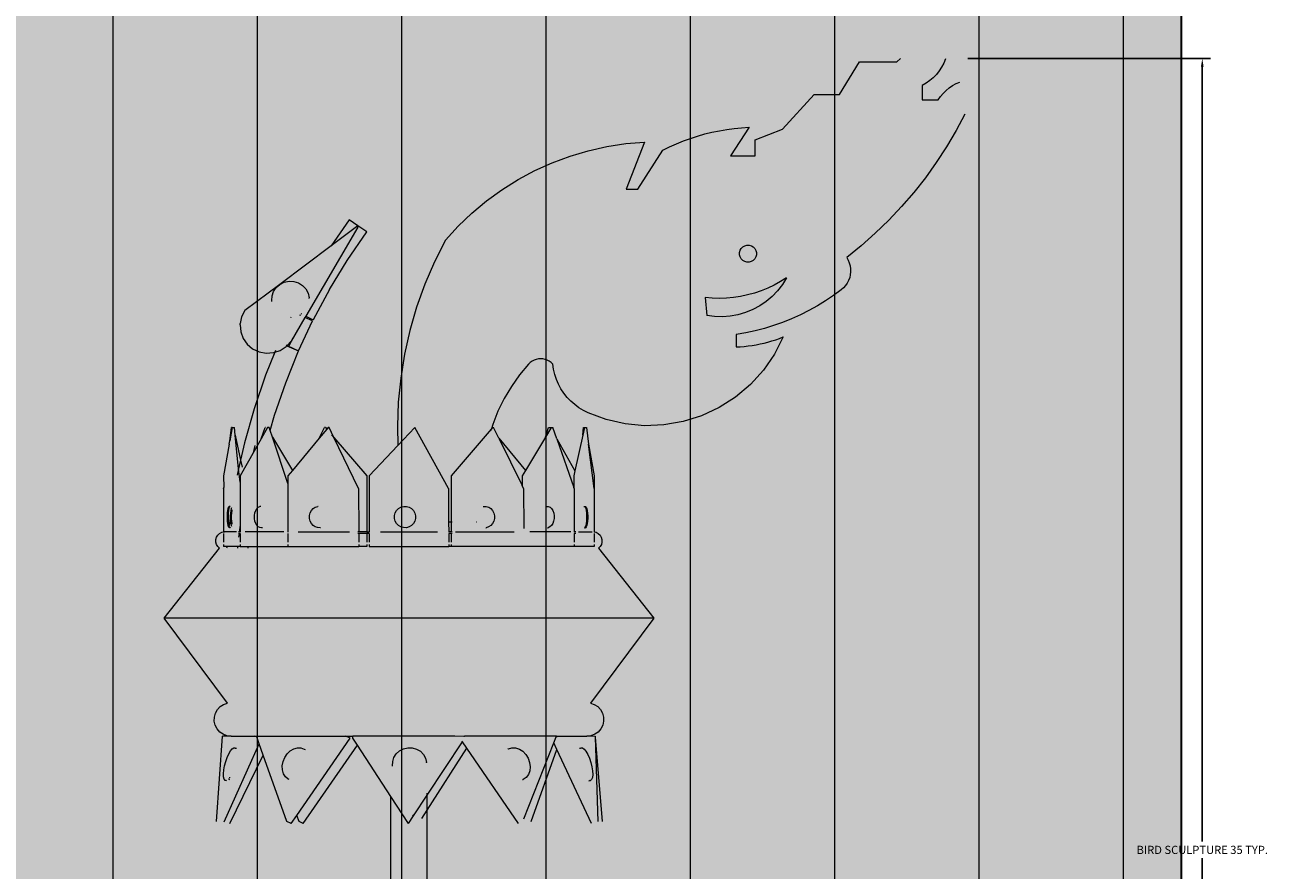
# Model space of a CAD drawing. Units: millimetres. Extents: x 446512 to 447461, y 70395 to 70610.
# Tile 36 of 39: x 447401 to 447428, y 70453 to 70472. Entities that reach past the tile are written whole.
import ezdxf

# ---------------------------------------------------------------- set-up
doc = ezdxf.new("R2010")
doc.units = ezdxf.units.MM
for name, color, linetype, lineweight in [('A-ANNO-DIMS', 2, 'Continuous', 18), ('A-FURN', 7, 'Continuous', 35), ('A-FURN-DECO', 8, 'Continuous', 13), ('A-FURN-PATT', 38, 'Continuous', 13)]:
    doc.layers.add(name, color=color, linetype=linetype, lineweight=lineweight)
doc.styles.get("Standard").update_dxf_attribs({"font": 'arial.ttf'})
doc.dimstyles.get("Standard").update_dxf_attribs({"dimtxt": 0.18, "dimasz": 0.18, "dimexe": 0.18, "dimexo": 0.0625, "dimgap": 0.09, "dimtad": 0, "dimtih": 1, "dimtoh": 1, "dimdec": 4, "dimzin": 0, "dimdsep": 46, "dimtxsty": 'Standard', "dimcen": 0.09, "dimadec": 0, "dimazin": 0, "dimtfac": 1, "dimtdec": 4, "dimtofl": 0, "dimtmove": 0, "dimatfit": 3, "dimfxl": 1, "dimtolj": 1, "dimtzin": 0, "dimarcsym": 0})

# ---------------------------------------------------------------- blocks, each defined once
blk = doc.blocks.new('DECO-SCULPTURE-BIRD')
for p, q in [((15.181, 34.03), (15.627, 34.749)), ((15.627, 34.749), (16.449, 34.749)), ((16.449, 34.749), (16.526, 34.819)), ((13.93, 33.268), (14.629, 34.03)), ((14.629, 34.03), (15.181, 34.03)), ((17.942, 33.598), (17.748, 33.234)), ((11.904, 33.064), (12.061, 33.115)), ((12.061, 33.115), (12.219, 33.16)), ((12.219, 33.16), (12.379, 33.199)), ((12.379, 33.199), (12.541, 33.233)), ((12.541, 33.233), (12.703, 33.261)), ((12.703, 33.261), (12.866, 33.283)), ((13.195, 33.309), (12.789, 32.676)), ((12.866, 33.283), (13.03, 33.299)), ((13.03, 33.299), (13.195, 33.309)), ((13.33, 33.029), (13.93, 33.268)), ((17.748, 33.234), (17.539, 32.879)), ((9.658, 32.793), (10.067, 32.884)), ((10.067, 32.884), (10.481, 32.948)), ((10.481, 32.948), (10.898, 32.983)), ((10.898, 32.983), (10.488, 31.945)), ((10.747, 31.945), (11.298, 32.806)), ((11.298, 32.806), (11.446, 32.878)), ((11.446, 32.878), (11.597, 32.946)), ((11.597, 32.946), (11.749, 33.008)), ((11.749, 33.008), (11.904, 33.064)), ((13.33, 32.676), (13.33, 33.029)), ((17.539, 32.879), (17.314, 32.533)), ((8.482, 32.355), (8.864, 32.528)), ((8.864, 32.528), (9.257, 32.674)), ((9.257, 32.674), (9.658, 32.793)), ((12.789, 32.676), (13.33, 32.676)), ((17.314, 32.533), (17.074, 32.198)), ((8.113, 32.157), (8.482, 32.355)), ((7.759, 31.935), (8.113, 32.157)), ((17.074, 32.198), (16.819, 31.874)), ((7.42, 31.689), (7.759, 31.935)), ((10.488, 31.945), (10.747, 31.945)), ((16.819, 31.874), (16.55, 31.562)), ((7.098, 31.42), (7.42, 31.689)), ((16.55, 31.562), (16.267, 31.262)), ((4.396, 31.274), (4.005, 30.703)), ((4.59, 31.141), (4.396, 31.274)), ((6.796, 31.131), (7.098, 31.42)), ((16.267, 31.262), (15.971, 30.975)), ((4.59, 31.11), (3.442, 29.152)), ((4.59, 31.141), (4.005, 30.703)), ((4.354, 30.38), (4.784, 31.008)), ((4.59, 31.11), (4.59, 31.141)), ((4.784, 31.008), (4.59, 31.141)), ((6.514, 30.821), (6.796, 31.131)), ((15.971, 30.975), (15.663, 30.701)), ((4.005, 30.703), (2.875, 29.852)), ((6.514, 30.821), (6.273, 30.344)), ((15.663, 30.701), (15.342, 30.442)), ((3.962, 29.736), (4.354, 30.38)), ((6.273, 30.344), (6.062, 29.854)), ((15.342, 30.442), (15.375, 30.385)), ((15.375, 30.385), (15.4, 30.324)), ((15.4, 30.324), (15.418, 30.261)), ((15.422, 30.065), (15.408, 30.001)), ((15.418, 30.261), (15.428, 30.196)), ((15.429, 30.13), (15.422, 30.065)), ((15.428, 30.196), (15.429, 30.13)), ((2.875, 29.852), (2.1, 29.278)), ((2.795, 29.783), (2.875, 29.852)), ((2.875, 29.852), (2.971, 29.899)), ((2.971, 29.899), (3.076, 29.921)), ((3.076, 29.921), (3.183, 29.915)), ((3.183, 29.915), (3.285, 29.883)), ((3.285, 29.883), (3.375, 29.827)), ((3.375, 29.827), (3.447, 29.75)), ((6.062, 29.854), (5.881, 29.351)), ((15.318, 29.827), (15.274, 29.778)), ((15.355, 29.881), (15.318, 29.827)), ((15.385, 29.939), (15.355, 29.881)), ((15.408, 30.001), (15.385, 29.939)), ((2.698, 29.494), (2.704, 29.597)), ((2.704, 29.597), (2.737, 29.696)), ((2.737, 29.696), (2.795, 29.783)), ((3.447, 29.75), (3.496, 29.657)), ((3.496, 29.657), (3.518, 29.556)), ((3.517, 29.541), (3.518, 29.556)), ((3.517, 29.541), (3.518, 29.538)), ((3.962, 29.736), (3.605, 29.071)), ((15.054, 29.609), (14.878, 29.491)), ((15.224, 29.735), (15.054, 29.609)), ((15.274, 29.778), (15.224, 29.735)), ((2.1, 29.278), (2.031, 29.139)), ((2.699, 29.49), (2.698, 29.494)), ((2.698, 29.476), (2.699, 29.49)), ((5.881, 29.351), (5.732, 28.838)), ((14.513, 29.277), (14.324, 29.181)), ((14.698, 29.38), (14.513, 29.277)), ((14.878, 29.491), (14.698, 29.38)), ((2.031, 29.139), (2.002, 28.989)), ((2.002, 28.958), (2.002, 28.989)), ((3.425, 29.125), (3.119, 28.602)), ((3.287, 28.392), (3.593, 29.046)), ((3.306, 29.18), (3.325, 29.171)), ((3.358, 29.194), (3.345, 29.201)), ((3.442, 29.152), (3.425, 29.125)), ((3.593, 29.046), (3.425, 29.125)), ((3.442, 29.152), (3.605, 29.071)), ((13.934, 29.015), (13.735, 28.944)), ((14.131, 29.094), (13.934, 29.015)), ((14.324, 29.181), (14.131, 29.094)), ((2.002, 28.958), (2.013, 28.805)), ((2.013, 28.805), (2.066, 28.66)), ((5.732, 28.838), (5.615, 28.317)), ((13.121, 28.783), (12.912, 28.746)), ((12.912, 28.746), (12.912, 28.476)), ((13.328, 28.828), (13.121, 28.783)), ((13.532, 28.882), (13.328, 28.828)), ((13.735, 28.944), (13.532, 28.882)), ((13.947, 28.695), (13.752, 28.315)), ((13.864, 28.663), (13.947, 28.695)), ((2.066, 28.66), (2.155, 28.533)), ((2.155, 28.533), (2.275, 28.433)), ((2.275, 28.433), (2.419, 28.366)), ((2.883, 28.399), (3.015, 28.486)), ((3.005, 28.509), (3.027, 28.499)), ((3.015, 28.486), (3.027, 28.499)), ((3.036, 28.509), (3.019, 28.518)), ((3.027, 28.499), (3.036, 28.509)), ((3.027, 28.499), (3.284, 28.387)), ((3.036, 28.509), (3.119, 28.602)), ((3.036, 28.509), (3.287, 28.392)), ((3.074, 28.492), (3.069, 28.481)), ((3.152, 28.659), (3.074, 28.492)), ((12.912, 28.476), (13.001, 28.48)), ((13.001, 28.48), (13.089, 28.487)), ((13.089, 28.487), (13.177, 28.496)), ((13.177, 28.496), (13.265, 28.508)), ((13.265, 28.508), (13.352, 28.523)), ((13.352, 28.523), (13.439, 28.54)), ((13.439, 28.54), (13.525, 28.559)), ((13.525, 28.559), (13.611, 28.581)), ((13.611, 28.581), (13.696, 28.606)), ((13.696, 28.606), (13.781, 28.633)), ((13.781, 28.633), (13.864, 28.663)), ((2.419, 28.366), (2.575, 28.337)), ((2.766, 28.36), (2.561, 27.852)), ((2.575, 28.337), (2.733, 28.349)), ((2.733, 28.349), (2.766, 28.36)), ((2.766, 28.36), (2.883, 28.399)), ((2.781, 28.395), (2.766, 28.36)), ((3.002, 27.688), (3.284, 28.387)), ((5.615, 28.317), (5.531, 27.79)), ((8.422, 28.162), (8.382, 28.133)), ((8.466, 28.185), (8.422, 28.162)), ((8.513, 28.202), (8.466, 28.185)), ((8.561, 28.212), (8.513, 28.202)), ((8.611, 28.216), (8.561, 28.212)), ((8.66, 28.212), (8.611, 28.216)), ((8.709, 28.202), (8.66, 28.212)), ((8.756, 28.185), (8.709, 28.202)), ((8.799, 28.162), (8.756, 28.185)), ((8.84, 28.133), (8.799, 28.162)), ((13.752, 28.315), (13.509, 27.964)), ((8.346, 28.098), (8.147, 27.859)), ((8.382, 28.133), (8.346, 28.098)), ((8.875, 28.098), (8.84, 28.133)), ((8.892, 27.984), (8.875, 28.098)), ((8.919, 27.871), (8.892, 27.984)), ((13.509, 27.964), (13.223, 27.648)), ((2.561, 27.852), (2.308, 27.114)), ((2.757, 26.974), (3.002, 27.688)), ((5.531, 27.79), (5.479, 27.259)), ((7.968, 27.605), (7.808, 27.338)), ((8.147, 27.859), (7.968, 27.605)), ((8.956, 27.761), (8.919, 27.871)), ((9.002, 27.655), (8.956, 27.761)), ((9.057, 27.553), (9.002, 27.655)), ((13.223, 27.648), (12.897, 27.372)), ((7.808, 27.338), (7.671, 27.059)), ((9.121, 27.456), (9.057, 27.553)), ((9.193, 27.366), (9.121, 27.456)), ((9.273, 27.282), (9.193, 27.366)), ((12.897, 27.372), (12.537, 27.142)), ((2.308, 27.114), (2.095, 26.364)), ((5.479, 27.259), (5.46, 26.725)), ((7.671, 27.059), (7.556, 26.77)), ((9.359, 27.205), (9.273, 27.282)), ((9.452, 27.136), (9.359, 27.205)), ((9.551, 27.075), (9.452, 27.136)), ((9.654, 27.023), (9.551, 27.075)), ((12.537, 27.142), (12.15, 26.961)), ((2.662, 26.638), (2.757, 26.974)), ((10.055, 26.875), (9.654, 27.023)), ((10.471, 26.78), (10.055, 26.875)), ((11.743, 26.833), (11.323, 26.759)), ((12.15, 26.961), (11.743, 26.833)), ((1.77, 26.41), (1.808, 26.703)), ((1.827, 26.703), (1.77, 26.41)), ((1.827, 26.703), (1.808, 26.703)), ((1.827, 26.703), (1.873, 26.703)), ((1.89, 26.535), (1.873, 26.703)), ((1.89, 26.535), (2.01, 25.987)), ((1.967, 25.795), (1.89, 26.535)), ((2.459, 26.45), (2.547, 26.703)), ((2.603, 26.703), (2.459, 26.45)), ((2.558, 26.703), (2.547, 26.703)), ((2.64, 26.703), (2.603, 26.703)), ((2.662, 26.638), (2.64, 26.703)), ((2.709, 26.493), (2.662, 26.638)), ((3.737, 26.466), (3.854, 26.703)), ((3.905, 26.667), (3.737, 26.466)), ((3.875, 26.703), (3.854, 26.703)), ((3.875, 26.703), (3.905, 26.667)), ((3.935, 26.703), (3.905, 26.667)), ((3.957, 26.703), (3.935, 26.703)), ((4.064, 26.48), (3.957, 26.703)), ((4.013, 26.541), (4.064, 26.48)), ((5.46, 26.725), (5.471, 26.308)), ((5.845, 26.703), (5.471, 26.308)), ((6.58, 25.364), (5.845, 26.703)), ((7.523, 26.665), (6.643, 25.636)), ((7.523, 26.665), (7.514, 26.636)), ((7.526, 26.673), (7.523, 26.665)), ((7.523, 26.665), (7.531, 26.655)), ((7.556, 26.77), (7.526, 26.673)), ((7.551, 26.703), (7.526, 26.673)), ((7.551, 26.703), (7.572, 26.703)), ((7.688, 26.466), (7.572, 26.703)), ((8.717, 26.493), (8.786, 26.703)), ((8.833, 26.686), (8.717, 26.493)), ((8.786, 26.703), (8.823, 26.703)), ((8.823, 26.703), (8.833, 26.686)), ((8.843, 26.703), (8.833, 26.686)), ((8.843, 26.703), (8.879, 26.703)), ((8.967, 26.45), (8.879, 26.703)), ((9.536, 26.535), (9.364, 25.75)), ((9.536, 26.535), (9.553, 26.703)), ((9.573, 26.703), (9.536, 26.535)), ((9.553, 26.703), (9.573, 26.703)), ((9.573, 26.703), (9.618, 26.703)), ((9.618, 26.703), (9.665, 26.337)), ((10.896, 26.742), (10.471, 26.78)), ((11.323, 26.759), (10.896, 26.742)), ((1.761, 26.337), (1.636, 25.636)), ((1.761, 26.337), (1.77, 26.41)), ((2.459, 26.45), (1.998, 25.636)), ((2.095, 26.364), (2.01, 25.987)), ((2.709, 26.493), (3.149, 25.76)), ((3.046, 25.467), (2.709, 26.493)), ((3.737, 26.466), (3.149, 25.76)), ((4.064, 26.48), (4.783, 25.636)), ((4.603, 25.364), (4.064, 26.48)), ((5.471, 26.308), (4.835, 25.636)), ((7.688, 26.466), (8.277, 25.76)), ((7.688, 26.466), (8.203, 25.423)), ((8.717, 26.493), (8.277, 25.76)), ((8.967, 26.45), (9.364, 25.75)), ((8.967, 26.45), (9.339, 25.38)), ((9.665, 26.337), (9.79, 25.636)), ((9.789, 25.364), (9.665, 26.337)), ((2.01, 25.987), (1.967, 25.795)), ((2.01, 25.987), (2.045, 25.829)), ((1.967, 25.795), (1.935, 25.655)), ((1.998, 25.499), (1.967, 25.795)), ((3.149, 25.76), (3.046, 25.636)), ((8.277, 25.76), (8.203, 25.636)), ((9.364, 25.75), (9.339, 25.636)), ((1.636, 25.636), (1.639, 25.38)), ((1.998, 25.636), (1.998, 25.499)), ((1.998, 25.499), (1.998, 24.41)), ((3.046, 25.636), (3.046, 25.467)), ((3.046, 25.467), (3.046, 24.397)), ((4.783, 25.636), (4.783, 24.41)), ((4.835, 25.636), (4.835, 24.41)), ((6.643, 25.636), (6.643, 24.617)), ((8.203, 25.636), (8.203, 25.423)), ((8.232, 25.364), (8.203, 25.423)), ((9.339, 25.636), (9.339, 25.38)), ((9.79, 25.636), (9.789, 25.364)), ((1.637, 25.364), (1.635, 24.407)), ((1.637, 25.364), (1.639, 25.38)), ((4.603, 25.364), (4.61, 24.41)), ((6.58, 25.364), (6.586, 24.617)), ((8.232, 25.364), (8.239, 24.482)), ((9.344, 25.364), (9.339, 25.38)), ((9.344, 25.364), (9.349, 24.41)), ((9.789, 25.364), (9.79, 24.407)), ((6.643, 24.617), (6.586, 24.617)), ((6.586, 24.617), (6.588, 24.41)), ((6.663, 24.617), (6.643, 24.617)), ((6.643, 24.617), (6.643, 24.41)), ((1.483, 24.287), (1.51, 24.333)), ((1.51, 24.333), (1.549, 24.371)), ((1.549, 24.371), (1.595, 24.397)), ((1.595, 24.397), (1.635, 24.407)), ((1.635, 24.407), (1.648, 24.41)), ((1.635, 24.407), (1.635, 24.397)), ((1.635, 24.371), (1.635, 24.182)), ((1.648, 24.41), (1.657, 24.41)), ((1.648, 24.41), (1.651, 24.41)), ((1.923, 24.41), (1.657, 24.41)), ((1.998, 24.41), (1.967, 24.41)), ((1.977, 24.371), (1.967, 24.29)), ((1.998, 24.367), (1.967, 24.367)), ((1.998, 24.556), (1.98, 24.397)), ((1.998, 24.41), (1.998, 24.397)), ((1.998, 24.371), (1.998, 24.367)), ((1.998, 24.367), (1.998, 24.182)), ((2.958, 24.41), (2.109, 24.41)), ((3.046, 24.371), (3.046, 24.182)), ((4.61, 24.41), (4.588, 24.41)), ((4.611, 24.367), (4.588, 24.367)), ((4.61, 24.41), (4.611, 24.397)), ((4.783, 24.41), (4.61, 24.41)), ((4.611, 24.371), (4.611, 24.367)), ((4.611, 24.367), (4.612, 24.182)), ((4.783, 24.367), (4.611, 24.367)), ((4.783, 24.41), (4.835, 24.41)), ((4.783, 24.41), (4.783, 24.397)), ((4.783, 24.371), (4.783, 24.367)), ((4.783, 24.367), (4.783, 24.182)), ((4.835, 24.367), (4.783, 24.367)), ((4.835, 24.41), (4.835, 24.397)), ((4.835, 24.371), (4.835, 24.367)), ((4.835, 24.367), (4.835, 24.182)), ((6.588, 24.41), (6.588, 24.397)), ((6.643, 24.41), (6.588, 24.41)), ((6.588, 24.371), (6.588, 24.367)), ((6.588, 24.367), (6.59, 24.182)), ((6.643, 24.367), (6.588, 24.367)), ((6.663, 24.41), (6.643, 24.41)), ((6.643, 24.41), (6.643, 24.397)), ((6.643, 24.371), (6.643, 24.367)), ((6.663, 24.367), (6.643, 24.367)), ((6.643, 24.367), (6.643, 24.182)), ((6.737, 24.41), (8.029, 24.41)), ((9.272, 24.41), (8.372, 24.41)), ((9.384, 24.41), (9.349, 24.41)), ((9.349, 24.41), (9.35, 24.397)), ((9.35, 24.371), (9.35, 24.367)), ((9.384, 24.367), (9.35, 24.367)), ((9.35, 24.367), (9.351, 24.182)), ((9.445, 24.41), (9.742, 24.41)), ((9.79, 24.407), (9.83, 24.397)), ((9.79, 24.407), (9.79, 24.397)), ((9.79, 24.371), (9.79, 24.182)), ((9.83, 24.397), (9.877, 24.371)), ((9.877, 24.371), (9.916, 24.333)), ((9.916, 24.333), (9.943, 24.287)), ((1.467, 24.182), (1.468, 24.235)), ((1.48, 24.13), (1.467, 24.182)), ((1.468, 24.235), (1.483, 24.287)), ((1.507, 24.083), (1.48, 24.13)), ((1.544, 24.044), (1.507, 24.083)), ((1.635, 24.13), (1.635, 24.083)), ((1.639, 24.083), (1.635, 24.083)), ((1.707, 24.083), (1.635, 24.083)), ((1.704, 24.059), (1.703, 24.044)), ((1.707, 24.083), (1.704, 24.059)), ((1.998, 24.083), (1.707, 24.083)), ((1.944, 24.083), (1.939, 24.044)), ((1.998, 24.13), (1.998, 24.083)), ((1.998, 24.083), (2.18, 24.083)), ((2.176, 24.044), (2.18, 24.083)), ((2.18, 24.083), (3.049, 24.083)), ((3.046, 24.13), (3.049, 24.083)), ((3.049, 24.083), (4.613, 24.083)), ((4.613, 24.13), (4.613, 24.083)), ((4.783, 24.083), (4.613, 24.083)), ((4.783, 24.13), (4.783, 24.083)), ((4.835, 24.13), (4.835, 24.083)), ((4.835, 24.083), (6.591, 24.083)), ((6.59, 24.13), (6.591, 24.083)), ((6.643, 24.083), (6.591, 24.083)), ((6.643, 24.13), (6.643, 24.083)), ((9.351, 24.083), (6.643, 24.083)), ((9.351, 24.13), (9.351, 24.083)), ((9.79, 24.083), (9.351, 24.083)), ((9.79, 24.13), (9.79, 24.083)), ((9.919, 24.083), (9.882, 24.044)), ((9.946, 24.13), (9.919, 24.083)), ((9.943, 24.287), (9.958, 24.235)), ((9.959, 24.182), (9.946, 24.13)), ((9.958, 24.235), (9.959, 24.182)), ((0.327, 22.505), (1.544, 24.044)), ((9.882, 24.044), (11.099, 22.505)), ((1.72, 20.641), (0.327, 22.505)), ((11.099, 22.505), (0.327, 22.505)), ((11.099, 22.505), (9.706, 20.641)), ((1.498, 20.496), (1.56, 20.562)), ((1.56, 20.562), (1.635, 20.611)), ((1.635, 20.611), (1.72, 20.641)), ((9.706, 20.641), (9.791, 20.611)), ((9.791, 20.611), (9.866, 20.562)), ((9.866, 20.562), (9.927, 20.496)), ((1.431, 20.239), (1.432, 20.329)), ((1.451, 20.152), (1.431, 20.239)), ((1.432, 20.329), (1.455, 20.417)), ((1.455, 20.417), (1.498, 20.496)), ((9.927, 20.496), (9.971, 20.417)), ((9.971, 20.417), (9.994, 20.329)), ((9.995, 20.239), (9.975, 20.152)), ((9.994, 20.329), (9.995, 20.239)), ((1.492, 20.071), (1.451, 20.152)), ((1.551, 20.003), (1.492, 20.071)), ((1.625, 19.952), (1.551, 20.003)), ((1.709, 19.92), (1.625, 19.952)), ((9.801, 19.952), (9.716, 19.92)), ((9.874, 20.003), (9.801, 19.952)), ((9.934, 20.071), (9.874, 20.003)), ((9.975, 20.152), (9.934, 20.071)), ((1.48, 18.035), (1.609, 19.909)), ((1.799, 19.909), (1.609, 19.909)), ((1.648, 18.028), (2.417, 19.746)), ((1.799, 19.909), (1.709, 19.92)), ((1.799, 19.909), (2.323, 19.909)), ((2.323, 19.909), (2.359, 19.909)), ((2.364, 19.896), (2.323, 19.909)), ((2.364, 19.896), (2.359, 19.909)), ((2.359, 19.909), (4.323, 19.909)), ((2.417, 19.746), (2.364, 19.896)), ((2.508, 19.49), (2.417, 19.746)), ((3.245, 18.169), (4.419, 19.866)), ((3.386, 17.993), (4.578, 19.714)), ((4.323, 19.909), (4.479, 19.909)), ((4.419, 19.866), (4.323, 19.909)), ((4.479, 19.866), (4.479, 19.909)), ((6.726, 19.909), (4.479, 19.909)), ((4.578, 19.714), (4.479, 19.866)), ((5.313, 18.586), (4.578, 19.714)), ((6.112, 18.612), (6.893, 19.784)), ((6.922, 19.907), (6.726, 19.909)), ((6.893, 19.784), (6.878, 19.805)), ((6.985, 19.65), (6.893, 19.784)), ((6.922, 19.907), (6.926, 19.909)), ((6.926, 19.909), (6.936, 19.909)), ((8.957, 19.909), (6.936, 19.909)), ((8.239, 18.093), (8.898, 19.762)), ((8.898, 19.762), (8.95, 19.895)), ((8.967, 19.615), (8.898, 19.762)), ((8.95, 19.895), (8.999, 19.909)), ((8.95, 19.895), (8.957, 19.909)), ((8.957, 19.909), (8.999, 19.909)), ((8.999, 19.909), (9.627, 19.909)), ((9.716, 19.92), (9.627, 19.909)), ((9.807, 19.907), (9.627, 19.909)), ((9.814, 19.909), (9.807, 19.907)), ((9.816, 19.893), (9.814, 19.909)), ((9.974, 18.035), (9.816, 19.893)), ((9.876, 18.035), (9.816, 19.893)), ((1.771, 17.993), (2.508, 19.49)), ((3.027, 18.035), (2.508, 19.49)), ((6.112, 18.284), (6.985, 19.65)), ((8.126, 17.993), (6.985, 19.65)), ((8.405, 18.035), (8.967, 19.615)), ((9.727, 17.993), (8.967, 19.615)), ((5.313, 11.612), (5.313, 18.586)), ((5.7, 17.993), (5.313, 18.586)), ((5.812, 18.161), (6.112, 18.612)), ((6.112, 18.612), (6.112, 18.655)), ((6.112, 18.284), (6.112, 18.612)), ((3.123, 17.993), (3.245, 18.169)), ((3.299, 18.035), (3.245, 18.169)), ((5.7, 17.993), (5.812, 18.161)), ((5.812, 18.161), (5.798, 18.182)), ((5.816, 18.155), (5.812, 18.161)), ((5.995, 18.101), (6.112, 18.284)), ((6.112, 11.612), (6.112, 18.284)), ((3.123, 17.993), (3.027, 18.035)), ((3.386, 17.993), (3.299, 18.035)), ((0, 0), (0, 11.612)), ((0, 11.612), (5.313, 11.612)), ((6.112, 11.612), (5.313, 11.612)), ((6.112, 11.612), (11.751, 11.612)), ((11.751, 0), (11.751, 11.612)), ((0, 0), (11.751, 0))]:
    blk.add_line(p, q)
blk = doc.blocks.new('*D5')
at = {"layer": 'A-ANNO-DIMS', "color": 0, "lineweight": -2, "transparency": 16777216}
for p, q in [((447421.309, 70471.106), (447426.65, 70471.106)), ((447426.47, 70470.926), (447426.47, 70453.88)), ((447426.47, 70436.468), (447426.47, 70453.514)), ((447421.309, 70436.288), (447426.65, 70436.288))]:
    blk.add_line(p, q, dxfattribs=at)
at = {"layer": 'A-ANNO-DIMS', "color": 0, "transparency": 16777216}
for points in [[(447426.44, 70470.926), (447426.5, 70470.926), (447426.47, 70471.106)], [(447426.44, 70436.468), (447426.5, 70436.468), (447426.47, 70436.288)]]:
    blk.add_solid(points, dxfattribs=at)
at = {"layer": 'Defpoints', "color": 0, "transparency": 16777216}
for p in [(447421.247, 70471.106), (447426.47, 70471.106), (447421.247, 70436.288)]:
    blk.add_point(p, dxfattribs=at)
at = {"layer": 'A-ANNO-DIMS', "color": 0, "transparency": 16777216, "insert": (447426.47, 70453.697), "char_height": 0.18, "attachment_point": 5}
blk.add_mtext('\\A1;BIRD SCULPTURE 35 TYP.', dxfattribs=at)

msp = doc.modelspace()

# ---------------------------------------------------------------- hatches: boundary and pattern name
at = {"layer": 'A-FURN-PATT'}
h = msp.add_hatch(dxfattribs=at)
h.set_pattern_fill('ANSI31', color=256, angle=45)
h.set_pattern_definition([(90, (127.5626, 0), (-3.175, 0), [])])
h.paths.add_polyline_path([(447426.0142, 70599.7147), (447365.4251, 70599.7147), (447365.4251, 70405.3145), (447426.0142, 70405.3145)])
h = msp.add_hatch(color=256, dxfattribs=at)
h.dxf.hatch_style = 1
h.paths.add_polyline_path([(447426.0142, 70502.5146), (447365.4251, 70502.5146), (447365.4251, 70436.2876), (447426.0142, 70436.2876)])

# ---------------------------------------------------------------- linework, layer by layer
at = {"layer": 'A-FURN'}
msp.add_line((447426.0142, 70405.3145), (447426.0142, 70599.7147), dxfattribs=at)
at = {"layer": 'A-FURN-DECO'}
for p, q in [((447420.8187, 70471.0982), (447420.7813, 70471.0063)), ((447420.6814, 70470.8351), (447420.6198, 70470.7573)), ((447420.7354, 70470.9183), (447420.6814, 70470.8351)), ((447420.7813, 70471.0063), (447420.7354, 70470.9183)), ((447420.395, 70470.5636), (447420.309, 70470.5141)), ((447420.476, 70470.621), (447420.395, 70470.5636)), ((447420.5511, 70470.6858), (447420.476, 70470.621)), ((447420.6198, 70470.7573), (447420.5511, 70470.6858)), ((447420.9776, 70470.5122), (447421.057, 70470.555)), ((447421.057, 70470.555), (447421.1401, 70470.5899)), ((447420.309, 70470.5141), (447420.309, 70470.1968)), ((447420.6616, 70470.1968), (447420.7119, 70470.2716)), ((447420.7119, 70470.2716), (447420.7693, 70470.3411)), ((447420.7693, 70470.3411), (447420.8331, 70470.4048)), ((447420.8331, 70470.4048), (447420.9027, 70470.462)), ((447420.9027, 70470.462), (447420.9776, 70470.5122)), ((447420.309, 70470.1968), (447420.6616, 70470.1968)), ((447416.3645, 70466.9653), (447416.4071, 70466.9896)), ((447416.4071, 70466.9896), (447416.4546, 70467.0021)), ((447416.4546, 70467.0021), (447416.5037, 70467.0018)), ((447416.5037, 70467.0018), (447416.551, 70466.9889)), ((447416.551, 70466.9889), (447416.5934, 70466.9641)), ((447416.2917, 70466.792), (447416.2919, 70466.841)), ((447416.3041, 70466.7445), (447416.2917, 70466.792)), ((447416.2919, 70466.841), (447416.3049, 70466.8884)), ((447416.3285, 70466.7019), (447416.3041, 70466.7445)), ((447416.3049, 70466.8884), (447416.3296, 70466.9308)), ((447416.3296, 70466.9308), (447416.3645, 70466.9653)), ((447416.5934, 70466.9641), (447416.628, 70466.9292)), ((447416.6515, 70466.7427), (447416.6268, 70466.7003)), ((447416.628, 70466.9292), (447416.6523, 70466.8866)), ((447416.6645, 70466.79), (447416.6515, 70466.7427)), ((447416.6523, 70466.8866), (447416.6647, 70466.8391)), ((447416.6647, 70466.8391), (447416.6645, 70466.79)), ((447416.363, 70466.667), (447416.3285, 70466.7019)), ((447416.4054, 70466.6422), (447416.363, 70466.667)), ((447416.4527, 70466.6293), (447416.4054, 70466.6422)), ((447416.5018, 70466.629), (447416.4527, 70466.6293)), ((447416.5493, 70466.6415), (447416.5018, 70466.629)), ((447416.5919, 70466.6658), (447416.5493, 70466.6415)), ((447416.6268, 70466.7003), (447416.5919, 70466.6658)), ((447417.1911, 70466.1996), (447417.0536, 70466.1239)), ((447417.324, 70466.2832), (447417.1911, 70466.1996)), ((447417.324, 70466.2832), (447417.2335, 70466.1359)), ((447416.4664, 70465.9057), (447416.3128, 70465.8731)), ((447416.6177, 70465.9472), (447416.4664, 70465.9057)), ((447416.7664, 70465.9975), (447416.6177, 70465.9472)), ((447416.9119, 70466.0565), (447416.7664, 70465.9975)), ((447417.0536, 70466.1239), (447416.9119, 70466.0565)), ((447417.128, 70465.9991), (447417.0087, 70465.874)), ((447417.2335, 70466.1359), (447417.128, 70465.9991)), ((447415.6875, 70465.8345), (447415.5311, 70465.8479)), ((447415.5311, 70465.8479), (447415.5696, 70465.4575)), ((447415.8444, 70465.8303), (447415.6875, 70465.8345)), ((447416.0013, 70465.8354), (447415.8444, 70465.8303)), ((447416.1576, 70465.8497), (447416.0013, 70465.8354)), ((447416.3128, 70465.8731), (447416.1576, 70465.8497)), ((447416.7342, 70465.665), (447416.5819, 70465.5832)), ((447416.877, 70465.7623), (447416.7342, 70465.665)), ((447417.0087, 70465.874), (447416.877, 70465.7623)), ((447406.4189, 70465.4177), (447406.4106, 70465.3999)), ((447415.7407, 70465.4334), (447415.5696, 70465.4575)), ((447415.9134, 70465.4274), (447415.7407, 70465.4334)), ((447416.0858, 70465.4396), (447415.9134, 70465.4274)), ((447416.2559, 70465.47), (447416.0858, 70465.4396)), ((447416.4219, 70465.518), (447416.2559, 70465.47)), ((447416.5819, 70465.5832), (447416.4219, 70465.518)), ((447405.6285, 70462.5935), (447405.5926, 70462.4346)), ((447405.0507, 70461.2367), (447405.062, 70461.2524)), ((447405.085, 70461.2524), (447405.062, 70461.2524)), ((447405.0738, 70461.2367), (447405.085, 70461.2524)), ((447405.705, 70461.2367), (447405.7405, 70461.2524)), ((447405.7594, 70461.2524), (447405.7405, 70461.2524)), ((447406.9584, 70461.2367), (447407.0106, 70461.2524)), ((447407.0218, 70461.2524), (447407.0106, 70461.2524)), ((447408.843, 70461.2367), (447408.9023, 70461.2524)), ((447408.9023, 70461.2524), (447408.9637, 70461.2522)), ((447408.9637, 70461.2522), (447409.0229, 70461.2362)), ((447410.6538, 70461.2524), (447410.6641, 70461.2524)), ((447410.6641, 70461.2524), (447410.7193, 70461.2522)), ((447410.7193, 70461.2522), (447410.7725, 70461.2362)), ((447412.0272, 70461.2524), (447412.0453, 70461.2524)), ((447412.0453, 70461.2524), (447412.0842, 70461.2522)), ((447412.0842, 70461.2522), (447412.1217, 70461.2362)), ((447412.8661, 70461.2524), (447412.8803, 70461.2522)), ((447412.8803, 70461.2522), (447412.889, 70461.2524)), ((447412.8803, 70461.2522), (447412.8941, 70461.2362)), ((447412.889, 70461.2524), (447412.9032, 70461.2522)), ((447412.9032, 70461.2522), (447412.9169, 70461.2362)), ((447405.0236, 70461.0506), (447405.0266, 70461.1098)), ((447405.0236, 70460.9893), (447405.0236, 70461.0506)), ((447405.0265, 70460.9299), (447405.0236, 70460.9893)), ((447405.0266, 70461.1098), (447405.0325, 70461.1629)), ((447405.0325, 70461.1629), (447405.0407, 70461.2061)), ((447405.0407, 70461.2061), (447405.0507, 70461.2367)), ((447405.0466, 70460.9893), (447405.0467, 70461.0506)), ((447405.0496, 70460.9299), (447405.0466, 70460.9893)), ((447405.0467, 70461.0506), (447405.0497, 70461.1098)), ((447405.0497, 70461.1098), (447405.0555, 70461.1629)), ((447405.0555, 70461.1629), (447405.0638, 70461.2061)), ((447405.0866, 70460.988), (447405.0636, 70460.8332)), ((447405.0638, 70461.2061), (447405.0738, 70461.2367)), ((447405.0902, 70461.1087), (447405.0866, 70461.0494)), ((447405.0866, 70461.0494), (447405.0866, 70460.988)), ((447405.0866, 70460.988), (447405.0903, 70460.9288)), ((447405.0973, 70461.1619), (447405.0902, 70461.1087)), ((447405.0983, 70461.1216), (447405.0902, 70461.1087)), ((447405.1073, 70461.2054), (447405.0973, 70461.1619)), ((447405.0973, 70461.1619), (447405.0983, 70461.1216)), ((447405.1131, 70461.2199), (447405.1073, 70461.2054)), ((447405.1144, 70461.2161), (447405.1073, 70461.2054)), ((447405.1131, 70461.1087), (447405.1094, 70461.0494)), ((447405.1094, 70461.0494), (447405.1095, 70460.988)), ((447405.1095, 70460.988), (447405.1132, 70460.9288)), ((447405.1202, 70461.1619), (447405.1131, 70461.1087)), ((447405.1234, 70461.176), (447405.1202, 70461.1619)), ((447405.6189, 70460.9893), (447405.619, 70461.0506)), ((447405.6283, 70460.9299), (447405.6189, 70460.9893)), ((447405.619, 70461.0506), (447405.6286, 70461.1098)), ((447405.6286, 70461.1098), (447405.6471, 70461.1629)), ((447405.6471, 70461.1629), (447405.6731, 70461.2061)), ((447405.6731, 70461.2061), (447405.705, 70461.2367)), ((447406.832, 70460.9893), (447406.8321, 70461.0506)), ((447406.8458, 70460.9299), (447406.832, 70460.9893)), ((447406.8321, 70461.0506), (447406.8463, 70461.1098)), ((447406.8463, 70461.1098), (447406.8734, 70461.1629)), ((447406.8734, 70461.1629), (447406.9116, 70461.2061)), ((447406.9116, 70461.2061), (447406.9584, 70461.2367)), ((447408.6993, 70460.9893), (447408.6994, 70461.0506)), ((447408.715, 70460.9299), (447408.6993, 70460.9893)), ((447408.6994, 70461.0506), (447408.7155, 70461.1098)), ((447408.7155, 70461.1098), (447408.7463, 70461.1629)), ((447408.7463, 70461.1629), (447408.7898, 70461.2061)), ((447408.7898, 70461.2061), (447408.843, 70461.2367)), ((447409.0229, 70461.2362), (447409.0759, 70461.2054)), ((447409.0759, 70461.2054), (447409.1192, 70461.1619)), ((447409.1192, 70461.1619), (447409.1497, 70461.1087)), ((447409.1653, 70460.988), (447409.1493, 70460.9288)), ((447409.1497, 70461.1087), (447409.1655, 70461.0494)), ((447409.1655, 70461.0494), (447409.1653, 70460.988)), ((447410.7725, 70461.2362), (447410.8203, 70461.2054)), ((447410.8203, 70461.2054), (447410.8592, 70461.1619)), ((447410.8592, 70461.1619), (447410.8867, 70461.1087)), ((447410.9006, 70460.988), (447410.8862, 70460.9288)), ((447410.8867, 70461.1087), (447410.9008, 70461.0494)), ((447410.9008, 70461.0494), (447410.9006, 70460.988)), ((447412.1217, 70461.2362), (447412.1553, 70461.2054)), ((447412.1553, 70461.2054), (447412.1827, 70461.1619)), ((447412.1827, 70461.1619), (447412.2021, 70461.1087)), ((447412.2119, 70460.988), (447412.2018, 70460.9288)), ((447412.2021, 70461.1087), (447412.212, 70461.0494)), ((447412.212, 70461.0494), (447412.2119, 70460.988)), ((447412.8941, 70461.2362), (447412.9064, 70461.2054)), ((447412.9064, 70461.2054), (447412.9164, 70461.1619)), ((447412.9164, 70461.1619), (447412.9235, 70461.1087)), ((447412.9169, 70461.2362), (447412.9292, 70461.2054)), ((447412.9271, 70460.988), (447412.9234, 70460.9288)), ((447412.9235, 70461.1087), (447412.9271, 70461.0494)), ((447412.9271, 70461.0494), (447412.9271, 70460.988)), ((447412.9292, 70461.2054), (447412.9392, 70461.1619)), ((447412.9392, 70461.1619), (447412.9463, 70461.1087)), ((447412.9499, 70460.988), (447412.9462, 70460.9288)), ((447412.9463, 70461.1087), (447412.95, 70461.0494)), ((447412.95, 70461.0494), (447412.9499, 70460.988)), ((447405.0323, 70460.8767), (447405.0265, 70460.9299)), ((447405.0405, 70460.8332), (447405.0323, 70460.8767)), ((447405.0505, 70460.8024), (447405.0405, 70460.8332)), ((447405.0554, 70460.8767), (447405.0496, 70460.9299)), ((447405.0617, 70460.7864), (447405.0505, 70460.8024)), ((447405.0636, 70460.8332), (447405.0554, 70460.8767)), ((447405.0733, 70460.7862), (447405.0617, 70460.7864)), ((447405.0736, 70460.8024), (447405.0636, 70460.8332)), ((447405.0848, 70460.7864), (447405.0733, 70460.7862)), ((447405.0848, 70460.7864), (447405.0736, 70460.8024)), ((447405.0964, 70460.7862), (447405.0848, 70460.7864)), ((447405.0903, 70460.9288), (447405.0975, 70460.8757)), ((447405.0975, 70460.8757), (447405.1075, 70460.8325)), ((447405.1075, 70460.8325), (447405.1131, 70460.8187)), ((447405.1132, 70460.9288), (447405.1203, 70460.8757)), ((447405.1203, 70460.8757), (447405.1234, 70460.8626)), ((447405.6466, 70460.8767), (447405.6283, 70460.9299)), ((447405.6725, 70460.8332), (447405.6466, 70460.8767)), ((447405.7043, 70460.8024), (447405.6725, 70460.8332)), ((447405.7398, 70460.7864), (447405.7043, 70460.8024)), ((447405.7766, 70460.7862), (447405.7398, 70460.7864)), ((447405.7954, 70460.7862), (447405.7766, 70460.7862)), ((447406.5808, 70460.6974), (447407.7107, 70460.6974)), ((447406.8727, 70460.8767), (447406.8458, 70460.9299)), ((447406.9107, 70460.8332), (447406.8727, 70460.8767)), ((447406.9574, 70460.8024), (447406.9107, 70460.8332)), ((447407.0095, 70460.7864), (447406.9574, 70460.8024)), ((447407.0635, 70460.7862), (447407.0095, 70460.7864)), ((447407.0747, 70460.7862), (447407.0635, 70460.7862)), ((447408.3934, 70460.6974), (447409.6432, 70460.6974)), ((447408.7455, 70460.8767), (447408.715, 70460.9299)), ((447408.7888, 70460.8332), (447408.7455, 70460.8767)), ((447408.8418, 70460.8024), (447408.7888, 70460.8332)), ((447408.9011, 70460.7864), (447408.8418, 70460.8024)), ((447408.9624, 70460.7862), (447408.9011, 70460.7864)), ((447409.0217, 70460.8019), (447408.9624, 70460.7862)), ((447409.0749, 70460.8325), (447409.0217, 70460.8019)), ((447409.1184, 70460.8757), (447409.0749, 70460.8325)), ((447409.1493, 70460.9288), (447409.1184, 70460.8757)), ((447410.5061, 70460.9095), (447410.4959, 70460.9094)), ((447410.7079, 70460.7862), (447410.7182, 70460.7862)), ((447410.7715, 70460.8019), (447410.7182, 70460.7862)), ((447410.8194, 70460.8325), (447410.7715, 70460.8019)), ((447410.8585, 70460.8757), (447410.8194, 70460.8325)), ((447410.8862, 70460.9288), (447410.8585, 70460.8757)), ((447412.0652, 70460.7862), (447412.0834, 70460.7862)), ((447412.121, 70460.8019), (447412.0834, 70460.7862)), ((447412.1547, 70460.8325), (447412.121, 70460.8019)), ((447412.1822, 70460.8757), (447412.1547, 70460.8325)), ((447412.2018, 70460.9288), (447412.1822, 70460.8757)), ((447412.8938, 70460.8019), (447412.8801, 70460.7862)), ((447412.8801, 70460.7862), (447412.9029, 70460.7862)), ((447412.9061, 70460.8325), (447412.8938, 70460.8019)), ((447412.9167, 70460.8019), (447412.9029, 70460.7862)), ((447412.9162, 70460.8757), (447412.9061, 70460.8325)), ((447412.9234, 70460.9288), (447412.9162, 70460.8757)), ((447412.929, 70460.8325), (447412.9167, 70460.8019)), ((447412.9391, 70460.8757), (447412.929, 70460.8325)), ((447412.9462, 70460.9288), (447412.9391, 70460.8757)), ((447405.0207, 70455.7328), (447405.0562, 70455.8135)), ((447405.0562, 70455.8135), (447405.0934, 70455.8787)), ((447405.0934, 70455.8787), (447405.1298, 70455.9238)), ((447405.1298, 70455.9238), (447405.1629, 70455.9457)), ((447405.1629, 70455.9457), (447405.1904, 70455.9431)), ((447405.1955, 70455.9366), (447405.1904, 70455.9431)), ((447405.1955, 70455.9366), (447405.223, 70455.9339)), ((447406.2867, 70455.7328), (447406.3407, 70455.8135)), ((447406.3407, 70455.8135), (447406.4081, 70455.8787)), ((447406.4081, 70455.8787), (447406.4841, 70455.9238)), ((447406.4841, 70455.9238), (447406.5636, 70455.9457)), ((447406.5636, 70455.9457), (447406.6412, 70455.9431)), ((447406.6412, 70455.9431), (447406.7142, 70455.9138)), ((447406.7142, 70455.9138), (447406.7323, 70455.9068)), ((447408.6885, 70455.7328), (447408.7399, 70455.8135)), ((447408.7399, 70455.8135), (447408.8112, 70455.8787)), ((447408.8112, 70455.8787), (447408.8976, 70455.9238)), ((447408.8976, 70455.9238), (447408.9931, 70455.9457)), ((447408.9931, 70455.9457), (447409.0912, 70455.9431)), ((447409.0912, 70455.9431), (447409.1853, 70455.916)), ((447409.1853, 70455.916), (447409.2689, 70455.8663)), ((447409.2689, 70455.8663), (447409.3363, 70455.7973)), ((447409.3363, 70455.7973), (447409.383, 70455.7139)), ((447411.1902, 70455.9146), (447411.2011, 70455.9178)), ((447411.2011, 70455.9178), (447411.2096, 70455.9238)), ((447411.2096, 70455.9238), (447411.2847, 70455.9457)), ((447411.2847, 70455.9457), (447411.3658, 70455.9431)), ((447411.3658, 70455.9431), (447411.4473, 70455.916)), ((447411.4473, 70455.916), (447411.5236, 70455.8663)), ((447411.5236, 70455.8663), (447411.5895, 70455.7973)), ((447411.5895, 70455.7973), (447411.6406, 70455.7139)), ((447412.7696, 70455.9366), (447412.8018, 70455.9457)), ((447412.7696, 70455.9366), (447412.7891, 70455.935)), ((447412.8018, 70455.9457), (447412.8349, 70455.9431)), ((447412.8349, 70455.9431), (447412.8728, 70455.916)), ((447412.8728, 70455.916), (447412.913, 70455.8663)), ((447412.913, 70455.8663), (447412.9528, 70455.7973)), ((447412.9528, 70455.7973), (447412.9893, 70455.7139)), ((447404.947, 70455.4549), (447404.9642, 70455.5471)), ((447404.9642, 70455.5471), (447404.9893, 70455.6419)), ((447404.9893, 70455.6419), (447405.0207, 70455.7328)), ((447406.232, 70455.5471), (447406.2496, 70455.6419)), ((447406.2352, 70455.4549), (447406.232, 70455.5471)), ((447406.2496, 70455.6419), (447406.2867, 70455.7328)), ((447408.6576, 70455.538), (447408.6579, 70455.5462)), ((447408.6579, 70455.5462), (447408.6604, 70455.6419)), ((447408.6604, 70455.6419), (447408.6885, 70455.7328)), ((447409.383, 70455.7139), (447409.4057, 70455.6217)), ((447409.4057, 70455.6126), (447409.4057, 70455.6217)), ((447411.6406, 70455.7139), (447411.6734, 70455.6217)), ((447411.6734, 70455.6217), (447411.6856, 70455.5269)), ((447411.6856, 70455.5269), (447411.6764, 70455.436)), ((447412.9893, 70455.7139), (447413.0201, 70455.6217)), ((447413.0201, 70455.6217), (447413.0432, 70455.5269)), ((447413.0432, 70455.5269), (447413.0569, 70455.436)), ((447404.939, 70455.3715), (447404.947, 70455.4549)), ((447404.9407, 70455.3026), (447404.939, 70455.3715)), ((447404.952, 70455.2529), (447404.9407, 70455.3026)), ((447404.9721, 70455.2258), (447404.952, 70455.2529)), ((447405.0524, 70455.2695), (447405.0639, 70455.2451)), ((447405.0639, 70455.2451), (447405.0694, 70455.2411)), ((447405.072, 70455.2953), (447405.0743, 70455.281)), ((447406.2587, 70455.3715), (447406.2352, 70455.4549)), ((447406.3012, 70455.3026), (447406.2587, 70455.3715)), ((447406.3596, 70455.2529), (447406.3012, 70455.3026)), ((447406.3803, 70455.2438), (447406.3596, 70455.2529)), ((447411.5226, 70455.2419), (447411.5142, 70455.2359)), ((447411.5226, 70455.2419), (447411.5336, 70455.2451)), ((447411.5977, 70455.2902), (447411.5336, 70455.2451)), ((447411.6464, 70455.3553), (447411.5977, 70455.2902)), ((447411.6764, 70455.436), (447411.6464, 70455.3553)), ((447413.036, 70455.2451), (447413.01, 70455.2231)), ((447413.0532, 70455.2902), (447413.036, 70455.2451)), ((447413.0603, 70455.3553), (447413.0532, 70455.2902)), ((447413.0569, 70455.436), (447413.0603, 70455.3553)), ((447404.9998, 70455.2233), (447404.9721, 70455.2258)), ((447405.0047, 70455.2167), (447404.9998, 70455.2233)), ((447412.9906, 70455.2247), (447412.9779, 70455.214)), ((447412.9779, 70455.214), (447413.01, 70455.2231))]:
    msp.add_line(p, q, dxfattribs=at)

# ---------------------------------------------------------------- block references
msp.add_blockref('DECO-SCULPTURE-BIRD', (447403.3053, 70436.2876), dxfattribs=at)

# ---------------------------------------------------------------- dimensions: what is measured, and where the dimension line sits
at = {"layer": 'A-ANNO-DIMS'}
dim = msp.add_linear_dim(base=(447426.4697, 70471.1062), p1=(447421.2469, 70436.2876), p2=(447421.2469, 70471.1062), angle=90, text='BIRD SCULPTURE <> TYP.', dimstyle='Standard', override={"dimdec": 0, "dimlfac": 1, "dimrnd": 0, "dimzin": 0, "dimdsep": 46, "dimlunit": 2}, dxfattribs=at)
dim.commit()
dim.dimension.update_dxf_attribs({"geometry": '*D5', "text_midpoint": (447426.4697, 70453.6969)})

doc.saveas('drawing.dxf')
